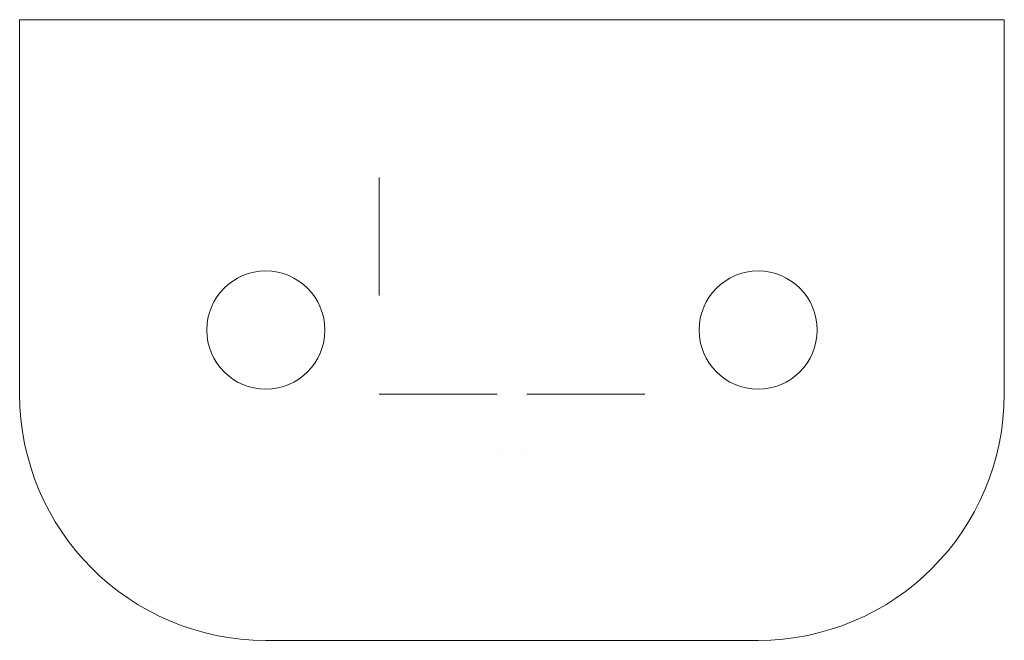
# Model space of a CAD drawing. Units: millimetres. Extents: x 2361 to 2850, y 0 to 1670.
# Tile 1 of 1: x 2361 to 2461, y 1606.9 to 1669.9. Entities that reach past the tile are written whole.
import ezdxf

# ---------------------------------------------------------------- set-up
doc = ezdxf.new("R2010")
doc.units = ezdxf.units.MM
doc.layers.add('M-CONS', color=8, linetype='Continuous', lineweight=18)

msp = doc.modelspace()

# ---------------------------------------------------------------- linework, layer by layer
at = {"layer": 'M-CONS'}
msp.add_line((2410.95, 1669.88), (2385.95, 1669.88), dxfattribs=at)
at = {"layer": 'M-CONS', "extrusion": (0, -1, 0)}
for p, q in [((2409.45, 1625.88, 114.95), (2409.45, 1625.88, 102.41)), ((2412.45, 1625.88, 114.95), (2412.45, 1625.88, 102.41))]:
    msp.add_line(p, q, dxfattribs=at)
at = {"layer": 'M-CONS'}
msp.add_lwpolyline([(2435.95, 1606.88, 0.41421), (2460.95, 1631.88), (2460.95, 1669.88), (2360.95, 1669.88), (2360.95, 1631.88, 0.41421), (2385.95, 1606.88)], format="xyb", close=True, dxfattribs=at)
at = {"layer": 'M-CONS', "extrusion": (0, -1, 0), "elevation": -1669.88}
msp.add_lwpolyline([(2386.81, 96.47), (2360.95, 0), (2410.95, 0), (2460.95, 0), (2435.1, 96.47)], dxfattribs=at)
at = {"layer": 'M-CONS', "extrusion": (0, -1, 0), "elevation": -1631.88}
for points in [[(2409.45, 114.95, 0.1283), (2397.45, 111.04), (2397.45, 138.95), (2409.45, 138.95)], [(2412.45, 114.95), (2412.45, 138.95), (2424.45, 138.95), (2424.45, 111.04, 0.1283)]]:
    msp.add_lwpolyline(points, format="xyb", close=True, dxfattribs=at)
at = {"layer": 'M-CONS', "extrusion": (0, -1, 0)}
for radius in [25, 12.5]:
    msp.add_circle((2410.95, 90, -1669.88), radius, dxfattribs=at)
at = {"layer": 'M-CONS', "extrusion": (-1, 0, 0)}
msp.add_circle((-1647.88, 125, -2397.45), 6, dxfattribs=at)
at = {"layer": 'M-CONS'}
for centre in [(2385.95, 1638.38), (2435.95, 1638.38)]:
    msp.add_circle(centre, 6, dxfattribs=at)

doc.saveas('drawing.dxf')
